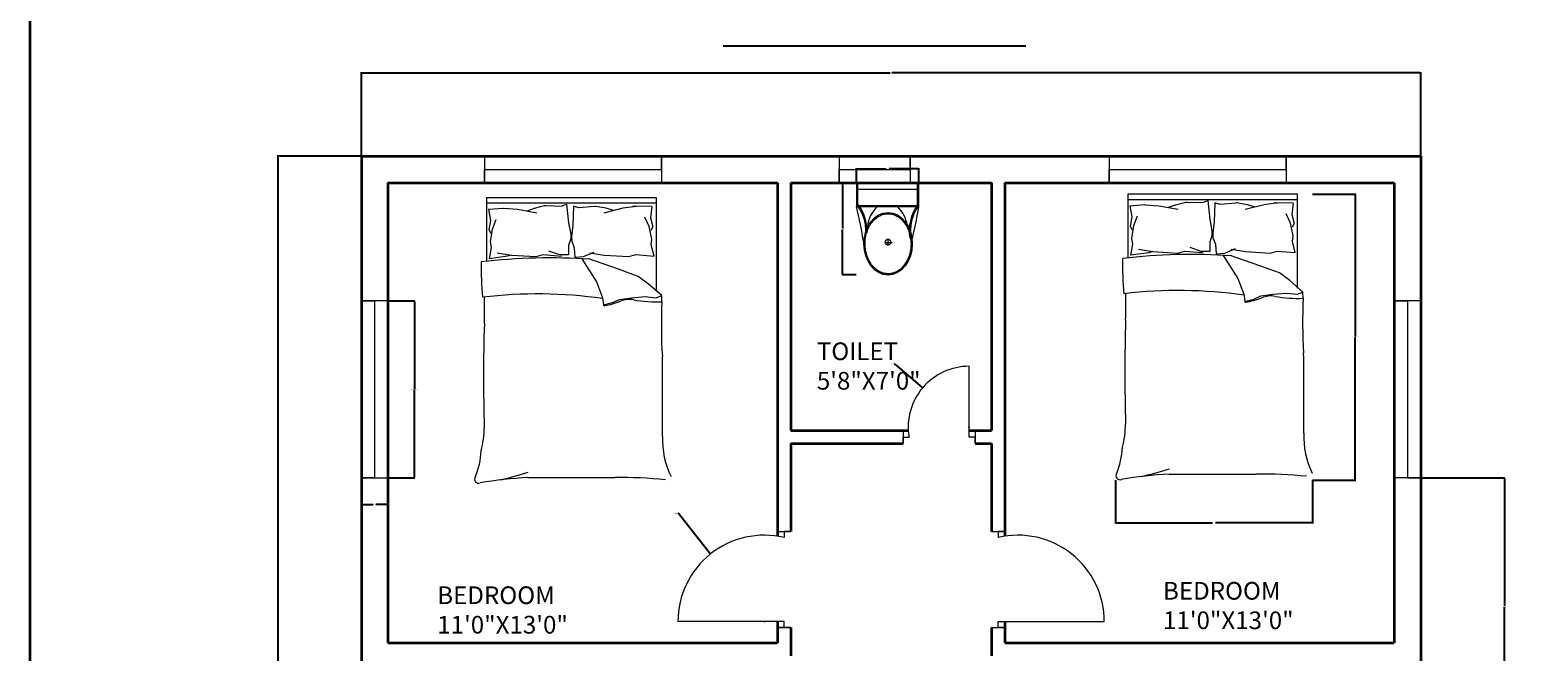
# Model space of a CAD drawing. Units: inches. Extents: x 1832 to 2989, y 1644 to 2902.
# Tile 3 of 8: x 1832 to 2343, y 2061 to 2272. Entities that reach past the tile are written whole.
import ezdxf

# ---------------------------------------------------------------- set-up
doc = ezdxf.new("R2010")
doc.units = ezdxf.units.IN
for name, color, linetype, lineweight in [('A-ANNO-DIMS', 2, 'Continuous', 18), ('A-ANNO-TEXT', 7, 'Continuous', 25), ('A-ANNO-TTLB', 7, 'Continuous', 35), ('A-AREA-IDEN', 7, 'Continuous', 18), ('A-DOOR', 3, 'Continuous', 18), ('A-FLOR-FIXT', 9, 'Continuous', 18), ('A-FURN', 8, 'Continuous', 18), ('A-GLAZ', 4, 'Continuous', 18), ('A-WALL', 7, 'Continuous', 35)]:
    doc.layers.add(name, color=color, linetype=linetype, lineweight=lineweight)
doc.styles.get("Standard").update_dxf_attribs({"font": 'arial.ttf'})
doc.dimstyles.get("Standard").update_dxf_attribs({"dimtxt": 0.18, "dimasz": 0.18, "dimexe": 0.18, "dimexo": 0.0625, "dimgap": 0.09, "dimtad": 0, "dimtih": 1, "dimtoh": 1, "dimdec": 4, "dimzin": 0, "dimdsep": 46, "dimtxsty": 'Standard', "dimcen": 0.09, "dimadec": 0, "dimazin": 0, "dimtfac": 1, "dimtdec": 4, "dimtofl": 0, "dimtmove": 0, "dimatfit": 3, "dimfxl": 1, "dimtolj": 1, "dimtzin": 0, "dimarcsym": 0})

# ---------------------------------------------------------------- blocks, each defined once
blk = doc.blocks.new('A$C31115884')
for p, q in [((258, 466), (258, 523)), ((283, 498), (223, 498)), ((0, 200), (0, 0)), ((520, 200), (0, 200)), ((10, 190), (10, 10)), ((510, 190), (10, 190)), ((510, 10), (510, 190)), ((520, 0), (520, 200)), ((510, 54), (0, 54)), ((10, 10), (510, 10)), ((0, 0), (520, 0))]:
    blk.add_line(p, q)
blk.add_circle((256, 496), 23.6)
for centre, radius, start, end in [((2778, -205), 2807, 165.4549, 171.7133), ((-295, 403), 365, 324.2091, 9.3499), ((-295, 403), 375, 324.2091, 9.3499), ((139, 406), 293, 315.8436, 2.6563), ((806, 403), 375, 179.2036, 215.7909), ((806, 403), 365, 170.6501, 215.7909), ((3237, 905), 2807, 188.2867, 194.5451), ((384, 406), 293, 190.2774, 224.1564)]:
    blk.add_arc(centre, radius, start, end)
blk.add_ellipse((256, 510), major_axis=(0, -261), ratio=0.772727)
blk.add_open_spline([(256, 259), (263, 259), (270, 260), (288, 262), (299, 265), (320, 273), (330, 278), (350, 291), (360, 299), (378, 316), (386, 326), (402, 347), (409, 358), (421, 383), (427, 395), (436, 422), (440, 436), (445, 465), (447, 480), (448, 509), (448, 524), (445, 553), (443, 568), (436, 596), (432, 610), (422, 636), (416, 649), (402, 672), (395, 683), (379, 703), (370, 712), (351, 728), (341, 735), (321, 746), (310, 751), (289, 757), (278, 759), (256, 761), (245, 761), (223, 757), (212, 754), (191, 746), (181, 741), (161, 728), (151, 720), (133, 703), (125, 693), (110, 672), (103, 660), (90, 636), (85, 623), (76, 596), (72, 582), (67, 553), (66, 538), (64, 509), (65, 494), (68, 465), (70, 450), (77, 422), (81, 408), (91, 382), (97, 370), (111, 346), (118, 335), (135, 316), (144, 307), (162, 291), (172, 284), (193, 273), (203, 269), (225, 262), (236, 260), (250, 259), (253, 259), (256, 259)], degree=3, knots=[0, 0, 0, 0, 0.110105, 0.110105, 0.285049, 0.285049, 0.459994, 0.459994, 0.634938, 0.634938, 0.809882, 0.809882, 0.984827, 0.984827, 1.159771, 1.159771, 1.334715, 1.334715, 1.50966, 1.50966, 1.684604, 1.684604, 1.859549, 1.859549, 2.034493, 2.034493, 2.209437, 2.209437, 2.384382, 2.384382, 2.559326, 2.559326, 2.73427, 2.73427, 2.909215, 2.909215, 3.084159, 3.084159, 3.259103, 3.259103, 3.434048, 3.434048, 3.608992, 3.608992, 3.783936, 3.783936, 3.958881, 3.958881, 4.133825, 4.133825, 4.30877, 4.30877, 4.483714, 4.483714, 4.658658, 4.658658, 4.833603, 4.833603, 5.008547, 5.008547, 5.183491, 5.183491, 5.358436, 5.358436, 5.53338, 5.53338, 5.708324, 5.708324, 5.883269, 5.883269, 6.058213, 6.058213, 6.233158, 6.233158, 6.283185, 6.283185, 6.283185, 6.283185])
blk = doc.blocks.new('BED-DOUBLE')
for p, q in [((4.17, 75.16), (4.17, 96.88)), ((4.17, 96.88), (61.46, 96.88)), ((4.17, 95.04), (61.46, 95.04)), ((4.67, 92.9), (5.36, 89.09)), ((4.68, 92.87), (9.81, 93.27)), ((9.81, 93.27), (9.93, 93.25)), ((9.93, 93.25), (14.52, 92.9)), ((14.52, 92.9), (21.1, 91.69)), ((17.81, 92.38), (20.24, 93.25)), ((20.24, 93.25), (23.7, 94.11)), ((23.7, 94.11), (24.09, 94.11)), ((24.09, 94.11), (29.42, 93.94)), ((29.42, 93.94), (31.15, 94.63)), ((31.15, 94.63), (31.84, 88.22)), ((33.54, 93.89), (33.25, 87.44)), ((35.31, 93.3), (33.54, 93.89)), ((40.62, 93.81), (35.31, 93.3)), ((41.01, 93.83), (40.62, 93.81)), ((44.52, 93.19), (41.01, 93.83)), ((50.25, 93.2), (43.75, 91.57)), ((47, 92.47), (44.52, 93.19)), ((54.8, 93.83), (50.25, 93.2)), ((60.08, 93.81), (53.6, 93.93)), ((53.6, 93.93), (54.8, 93.83)), ((60.08, 93.81), (59.62, 89.96)), ((61.46, 96.88), (61.46, 64.97)), ((5.36, 89.09), (4.84, 85.97)), ((6.06, 86.14), (7.27, 89.43)), ((31.84, 88.22), (32.54, 84.41)), ((33.25, 87.44), (32.8, 83.6)), ((59.12, 86.98), (57.7, 90.19)), ((60.08, 82.7), (59.12, 86.98)), ((59.62, 89.96), (60.34, 86.88)), ((60.34, 86.88), (59.72, 85.63)), ((4.84, 85.97), (5.54, 84.75)), ((5.36, 81.81), (6.06, 86.14)), ((5.71, 79.9), (5.36, 81.81)), ((32.54, 82.85), (31.84, 80.59)), ((32.54, 84.41), (32.54, 82.85)), ((32.8, 83.6), (32.89, 82.04)), ((32.89, 82.04), (33.73, 79.83)), ((59.85, 80.77), (60.08, 82.7)), ((5.02, 76.09), (5.71, 79.9)), ((11.13, 76.95), (5.02, 76.09)), ((7.65, 78.14), (12.49, 77.34)), ((12.49, 77.34), (11.13, 76.95)), ((12.49, 77.34), (20.89, 76.82)), ((20.89, 76.82), (23.24, 77.49)), ((23.24, 77.49), (29.39, 77.01)), ((28.9, 77.38), (25.13, 78.69)), ((31.84, 77.38), (28.9, 77.38)), ((31.84, 80.59), (31.84, 77.38)), ((33.73, 79.83), (33.93, 76.62)), ((33.93, 76.62), (36.87, 76.81)), ((36.87, 76.81), (40.55, 78.35)), ((39.04, 78.14), (43.88, 77.34)), ((43.88, 77.34), (52.28, 76.82)), ((52.28, 76.82), (54.63, 77.49)), ((54.63, 77.49), (60.78, 77.01)), ((60.78, 77.01), (59.85, 80.77)), ((36.28, 76.04), (41.3, 68.25)), ((48.73, 72.52), (38.73, 76.04)), ((55.41, 70.11), (48.73, 72.52)), ((41.3, 68.25), (43.34, 62.87)), ((58.94, 67.51), (55.41, 70.11)), ((63.38, 63.61), (58.94, 67.51)), ((43.34, 62.87), (43.72, 60.46)), ((46.69, 61.2), (49.1, 62.31)), ((49.1, 62.31), (53.18, 62.87)), ((53.18, 62.87), (57.83, 63.24)), ((57.83, 63.24), (61.54, 62.87)), ((61.54, 62.87), (63.38, 63.61)), ((63.48, 61.52), (63.38, 63.61, 4.64)), ((43.72, 60.46), (46.69, 61.2)), ((18.06, 1.87), (47.57, 1.87))]:
    blk.add_line(p, q)
for centre, radius, start, end in [((102.1, 72.78), 99.87, 178.7218, 185.604), ((25.61, -121.38), 197.77, 86.0865, 96.7821), ((21.29, -90.53), 154.68, 81.7845, 96.9006), ((-200.58, 59.5), 203.94, 358.4762, 1.0082), ((37.35, 95.1), 35.55, 280.6617, 289.8806), ((52.44, 54.84), 7.46, 78.6608, 113.7384), ((61.54, 104.86), 43.38, 259.8763, 272.5657), ((218.51, 53.34), 155.25, 176.9791, 183.8365), ((43.92, 60.38), 0.221, 160.2464, 271.1377), ((581.23, 36.2), 578.22, 178.22771, 181.71854), ((-5405.34, 15.57), 5469.02, 0.00217, 0.28689), ((-32.25, 19.53), 35.53, 346.0648, 358.9113), ((91.3, 14.55), 27.65, 177.4714, 206.4681), ((-25.96, 12.63), 28.25, 337.9751, 356.652), ((1.31, 1.31), 1.31, 146.1736, 293.4781), ((25.69, -143.9), 145.97, 92.9958, 99.4091), ((-20.64, 125.3), 127.63, 283.3832, 287.7053), ((49.34, -157.61), 159.5, 84.4998, 90.6351)]:
    blk.add_arc(centre, radius, start, end)
blk = doc.blocks.new('WIN-PLAN-60IN')
for p, q in [((0, 9), (0, 0)), ((60, 4.5), (60, 9)), ((60, 9), (60, 0)), ((0, 0), (0, 4.5)), ((0, 4.5), (60, 4.5))]:
    blk.add_line(p, q)
blk = doc.blocks.new('WIN-PLAN-60IN-2')
for p, q in [((9, 60), (0, 60)), ((0, 60), (4.5, 60)), ((4.5, 60), (4.5, 0)), ((4.5, 0), (0, 0)), ((0, 0), (9, 0))]:
    blk.add_line(p, q)
blk = doc.blocks.new('WIN-PLAN-24IN')
for p, q in [((0, 9), (0, 0)), ((24, 4.5), (24, 9)), ((24, 9), (24, 0)), ((0, 0), (0, 4.5)), ((0, 4.5), (24, 4.5))]:
    blk.add_line(p, q)
blk = doc.blocks.new('DOOR-PLAN-BEDROOM-L')
for p, q in [((33.75, 32.55), (38.25, 32.55)), ((38.25, 32.55), (36, 32.55)), ((36, 32.55), (36, 30.55)), ((36, 2), (0, 2)), ((33.75, 0), (38.25, 0)), ((38.25, 0), (33.75, 0)), ((33.75, 0), (36, 0)), ((36, 0), (36, 2))]:
    blk.add_line(p, q)
blk.add_arc((29.32, 2), 29.32, 76.8389, 180)
blk = doc.blocks.new('DOOR-PLAN-BATH')
for p, q in [((22.39, 2.25), (22.39, 26.25)), ((0, 4.5), (0, 0)), ((0, 0), (0, 2.25)), ((0, 2.25), (2, 2.25)), ((24.39, 2.25), (22.39, 2.25)), ((24.39, 4.5), (24.39, 0)), ((24.39, 0), (24.39, 2.25))]:
    blk.add_line(p, q)
blk.add_arc((22.39, 5.59), 20.66, 90, 189.2955)
blk = doc.blocks.new('DOOR-PLAN-BEDROOM-R')
for p, q in [((0, 32.55), (4.5, 32.55)), ((4.5, 32.55), (2.25, 32.55)), ((2.25, 32.55), (2.25, 30.55)), ((0, 0), (4.5, 0)), ((2.25, 0), (2.25, 2)), ((2.25, 2), (38.25, 2)), ((4.5, 0), (2.25, 0))]:
    blk.add_line(p, q)
blk.add_arc((8.93, 2), 29.32, 0, 103.1611)
blk = doc.blocks.new('*D25')
at = {"layer": 'A-ANNO-DIMS', "color": 0, "lineweight": -2, "transparency": 16777216}
for p, q in [((2266.19, 2216.33), (2280.86, 2216.33)), ((2280.68, 2216.15), (2280.68, 2168.02)), ((2280.68, 2119.51), (2280.68, 2167.65)), ((2266.19, 2119.33), (2280.86, 2119.33))]:
    blk.add_line(p, q, dxfattribs=at)
at = {"layer": 'A-ANNO-DIMS', "color": 0, "transparency": 16777216}
for points in [[(2280.65, 2216.15), (2280.71, 2216.15), (2280.68, 2216.33)], [(2280.65, 2119.51), (2280.71, 2119.51), (2280.68, 2119.33)]]:
    blk.add_solid(points, dxfattribs=at)
at = {"layer": 'Defpoints', "color": 0, "transparency": 16777216}
for p in [(2266.13, 2216.33), (2280.68, 2216.33), (2266.13, 2119.33)]:
    blk.add_point(p, dxfattribs=at)
at = {"layer": 'A-ANNO-DIMS', "color": 0, "transparency": 16777216, "insert": (2280.68, 2167.83), "char_height": 0.18, "attachment_point": 5}
blk.add_mtext('\\A1;DOUBLE BED 97 TYP.', dxfattribs=at)
blk = doc.blocks.new('*D26')
at = {"layer": 'A-ANNO-DIMS', "color": 0, "lineweight": -2, "transparency": 16777216}
for p, q in [((2199.47, 2119.27), (2199.47, 2104.6)), ((2266.13, 2119.27), (2266.13, 2104.6)), ((2199.65, 2104.78), (2232.27, 2104.78)), ((2265.95, 2104.78), (2233.33, 2104.78))]:
    blk.add_line(p, q, dxfattribs=at)
at = {"layer": 'A-ANNO-DIMS', "color": 0, "transparency": 16777216}
for points in [[(2199.65, 2104.81), (2199.65, 2104.75), (2199.47, 2104.78)], [(2265.95, 2104.81), (2265.95, 2104.75), (2266.13, 2104.78)]]:
    blk.add_solid(points, dxfattribs=at)
at = {"layer": 'Defpoints', "color": 0, "transparency": 16777216}
for p in [(2199.47, 2119.33), (2266.13, 2119.33), (2266.13, 2104.78)]:
    blk.add_point(p, dxfattribs=at)
at = {"layer": 'A-ANNO-DIMS', "color": 0, "transparency": 16777216, "insert": (2232.8, 2104.78), "char_height": 0.18, "attachment_point": 5}
blk.add_mtext('\\A1;67 TYP.', dxfattribs=at)
blk = doc.blocks.new('*D27')
at = {"layer": 'A-ANNO-DIMS', "color": 0, "lineweight": -2, "transparency": 16777216}
for p, q in [((2111.57, 2220.17), (2106.76, 2220.17)), ((2106.94, 2219.99), (2106.94, 2204.7)), ((2106.94, 2189.05), (2106.94, 2204.34)), ((2111.57, 2188.87), (2106.76, 2188.87))]:
    blk.add_line(p, q, dxfattribs=at)
at = {"layer": 'A-ANNO-DIMS', "color": 0, "transparency": 16777216}
for points in [[(2106.91, 2219.99), (2106.97, 2219.99), (2106.94, 2220.17)], [(2106.91, 2189.05), (2106.97, 2189.05), (2106.94, 2188.87)]]:
    blk.add_solid(points, dxfattribs=at)
at = {"layer": 'Defpoints', "color": 0, "transparency": 16777216}
for p in [(2111.64, 2220.17), (2106.94, 2188.87), (2111.64, 2188.87)]:
    blk.add_point(p, dxfattribs=at)
at = {"layer": 'A-ANNO-DIMS', "color": 0, "transparency": 16777216, "insert": (2106.94, 2204.52), "char_height": 0.18, "attachment_point": 5}
blk.add_mtext('\\A1;WC 31 TYP.', dxfattribs=at)
blk = doc.blocks.new('*D28')
at = {"layer": 'A-ANNO-DIMS', "color": 0, "lineweight": -2, "transparency": 16777216}
for p, q in [((2111.64, 2220.24), (2111.64, 2225.05)), ((2111.82, 2224.87), (2121.67, 2224.87)), ((2132.58, 2224.87), (2122.73, 2224.87)), ((2132.76, 2220.24), (2132.76, 2225.05))]:
    blk.add_line(p, q, dxfattribs=at)
at = {"layer": 'A-ANNO-DIMS', "color": 0, "transparency": 16777216}
for points in [[(2111.82, 2224.9), (2111.82, 2224.84), (2111.64, 2224.87)], [(2132.58, 2224.9), (2132.58, 2224.84), (2132.76, 2224.87)]]:
    blk.add_solid(points, dxfattribs=at)
at = {"layer": 'Defpoints', "color": 0, "transparency": 16777216}
for p in [(2111.64, 2224.87), (2111.64, 2220.17), (2132.76, 2220.17)]:
    blk.add_point(p, dxfattribs=at)
at = {"layer": 'A-ANNO-DIMS', "color": 0, "transparency": 16777216, "insert": (2122.2, 2224.87), "char_height": 0.18, "attachment_point": 5}
blk.add_mtext('\\A1;21 TYP.', dxfattribs=at)
blk = doc.blocks.new('*D51')
at = {"layer": 'A-ANNO-DIMS', "color": 0, "lineweight": -2, "transparency": 16777216}
for p, q in [((1952.95, 2180.08), (1962.07, 2180.08)), ((1961.89, 2179.9), (1961.89, 2150.27)), ((1961.89, 2120.26), (1961.89, 2149.9)), ((1952.95, 2120.08), (1962.07, 2120.08))]:
    blk.add_line(p, q, dxfattribs=at)
at = {"layer": 'A-ANNO-DIMS', "color": 0, "transparency": 16777216}
for points in [[(1961.86, 2179.9), (1961.92, 2179.9), (1961.89, 2180.08)], [(1961.86, 2120.26), (1961.92, 2120.26), (1961.89, 2120.08)]]:
    blk.add_solid(points, dxfattribs=at)
at = {"layer": 'Defpoints', "color": 0, "transparency": 16777216}
for p in [(1952.89, 2180.08), (1961.89, 2180.08), (1952.89, 2120.08)]:
    blk.add_point(p, dxfattribs=at)
at = {"layer": 'A-ANNO-DIMS', "color": 0, "transparency": 16777216, "insert": (1961.89, 2150.08), "char_height": 0.18, "attachment_point": 5}
blk.add_mtext('\\A1;SIDE WINDOW 60 TYP.', dxfattribs=at)
blk = doc.blocks.new('*D52')
at = {"layer": 'A-ANNO-DIMS', "color": 0, "lineweight": -2, "transparency": 16777216}
for p, q in [((1943.89, 2120.02), (1943.89, 2110.9)), ((1952.89, 2120.02), (1952.89, 2110.9)), ((1944.07, 2111.08), (1947.93, 2111.08)), ((1952.71, 2111.08), (1948.85, 2111.08))]:
    blk.add_line(p, q, dxfattribs=at)
at = {"layer": 'A-ANNO-DIMS', "color": 0, "transparency": 16777216}
for points in [[(1944.07, 2111.11), (1944.07, 2111.05), (1943.89, 2111.08)], [(1952.71, 2111.11), (1952.71, 2111.05), (1952.89, 2111.08)]]:
    blk.add_solid(points, dxfattribs=at)
at = {"layer": 'Defpoints', "color": 0, "transparency": 16777216}
for p in [(1943.89, 2120.08), (1952.89, 2120.08), (1952.89, 2111.08)]:
    blk.add_point(p, dxfattribs=at)
at = {"layer": 'A-ANNO-DIMS', "color": 0, "transparency": 16777216, "insert": (1948.39, 2111.08), "char_height": 0.18, "attachment_point": 5}
blk.add_mtext('\\A1;9 TYP.', dxfattribs=at)
blk = doc.blocks.new('*D71')
at = {"layer": 'A-ANNO-DIMS', "color": 0, "lineweight": -2, "transparency": 16777216}
for p, q in [((1943.89, 2229.24), (1943.89, 2257.65)), ((1944.07, 2257.47), (2123.1, 2257.47)), ((2302.71, 2257.47), (2123.68, 2257.47)), ((2302.89, 2229.24), (2302.89, 2257.65))]:
    blk.add_line(p, q, dxfattribs=at)
at = {"layer": 'A-ANNO-DIMS', "color": 0, "transparency": 16777216}
for points in [[(1944.07, 2257.5), (1944.07, 2257.44), (1943.89, 2257.47)], [(2302.71, 2257.5), (2302.71, 2257.44), (2302.89, 2257.47)]]:
    blk.add_solid(points, dxfattribs=at)
at = {"layer": 'Defpoints', "color": 0, "transparency": 16777216}
for p in [(2302.89, 2257.47), (1943.89, 2229.17), (2302.89, 2229.17)]:
    blk.add_point(p, dxfattribs=at)
at = {"layer": 'A-ANNO-DIMS', "color": 0, "transparency": 16777216, "insert": (2123.39, 2257.47), "char_height": 0.18, "attachment_point": 5}
blk.add_mtext('\\A1;359', dxfattribs=at)
blk = doc.blocks.new('*D72')
at = {"layer": 'A-ANNO-DIMS', "color": 0, "lineweight": -2, "transparency": 16777216}
for p, q in [((1943.83, 2229.17), (1915.41, 2229.17)), ((1915.59, 2228.99), (1915.59, 1975.53)), ((1915.59, 1721.7), (1915.59, 1975.17)), ((2089.33, 1721.52), (1915.41, 1721.52))]:
    blk.add_line(p, q, dxfattribs=at)
at = {"layer": 'A-ANNO-DIMS', "color": 0, "transparency": 16777216}
for points in [[(1915.56, 2228.99), (1915.62, 2228.99), (1915.59, 2229.17)], [(1915.56, 1721.7), (1915.62, 1721.7), (1915.59, 1721.52)]]:
    blk.add_solid(points, dxfattribs=at)
at = {"layer": 'Defpoints', "color": 0, "transparency": 16777216}
for p in [(1915.59, 2229.17), (1943.89, 2229.17), (2089.39, 1721.52)]:
    blk.add_point(p, dxfattribs=at)
at = {"layer": 'A-ANNO-DIMS', "color": 0, "transparency": 16777216, "insert": (1915.59, 1975.35), "char_height": 0.18, "attachment_point": 5}
blk.add_mtext('\\A1;507.6', dxfattribs=at)
blk = doc.blocks.new('*D74')
at = {"layer": 'A-ANNO-DIMS', "color": 0, "lineweight": -2, "transparency": 16777216}
for p, q in [((2302.95, 2120.08), (2331.37, 2120.08)), ((2331.19, 2119.9), (2331.19, 2076.73)), ((2331.19, 2033.19), (2331.19, 2076.36)), ((2302.95, 2033.01), (2331.37, 2033.01))]:
    blk.add_line(p, q, dxfattribs=at)
at = {"layer": 'A-ANNO-DIMS', "color": 0, "transparency": 16777216}
for points in [[(2331.16, 2119.9), (2331.22, 2119.9), (2331.19, 2120.08)], [(2331.16, 2033.19), (2331.22, 2033.19), (2331.19, 2033.01)]]:
    blk.add_solid(points, dxfattribs=at)
at = {"layer": 'Defpoints', "color": 0, "transparency": 16777216}
for p in [(2302.89, 2120.08), (2331.19, 2120.08), (2302.89, 2033.01)]:
    blk.add_point(p, dxfattribs=at)
at = {"layer": 'A-ANNO-DIMS', "color": 0, "transparency": 16777216, "insert": (2331.19, 2076.55), "char_height": 0.18, "attachment_point": 5}
blk.add_mtext('\\A1;87.08', dxfattribs=at)
blk = doc.blocks.new('*D122')
at = {"layer": 'A-ANNO-DIMS', "color": 0, "lineweight": -2, "transparency": 16777216}
for p, q in [((2051.13, 2108.07), (2051.31, 2108.07)), ((2051.31, 2108.07), (2062.13, 2094.43)), ((2080.37, 2071.31), (2080.55, 2071.31)), ((2080.46, 2071.22), (2080.46, 2071.4))]:
    blk.add_line(p, q, dxfattribs=at)
at = {"layer": 'A-ANNO-DIMS', "color": 0, "transparency": 16777216}
blk.add_solid([(2062.15, 2094.45), (2062.11, 2094.41), (2062.24, 2094.29)], dxfattribs=at)
at = {"layer": 'Defpoints', "color": 0, "transparency": 16777216}
for p in [(2062.24, 2094.29), (2080.46, 2071.31)]:
    blk.add_point(p, dxfattribs=at)
at = {"layer": 'A-ANNO-DIMS', "color": 0, "transparency": 16777216, "insert": (2050.38, 2108.07), "char_height": 0.18, "attachment_point": 5}
blk.add_mtext('\\A1;2X R29.323', dxfattribs=at)
blk = doc.blocks.new('*D126')
at = {"layer": 'A-ANNO-DIMS', "color": 0, "lineweight": -2, "transparency": 16777216}
for p, q in [((2124.48, 2158.67), (2124.66, 2158.67)), ((2124.66, 2158.67), (2133.97, 2150.76)), ((2149.77, 2137.26), (2149.95, 2137.26)), ((2149.86, 2137.17), (2149.86, 2137.35))]:
    blk.add_line(p, q, dxfattribs=at)
at = {"layer": 'A-ANNO-DIMS', "color": 0, "transparency": 16777216}
blk.add_solid([(2133.99, 2150.78), (2133.95, 2150.73), (2134.11, 2150.64)], dxfattribs=at)
at = {"layer": 'Defpoints', "color": 0, "transparency": 16777216}
for p in [(2134.11, 2150.64), (2149.86, 2137.26)]:
    blk.add_point(p, dxfattribs=at)
at = {"layer": 'A-ANNO-DIMS', "color": 0, "transparency": 16777216, "insert": (2123.93, 2158.67), "char_height": 0.18, "attachment_point": 5}
blk.add_mtext('\\A1;R20.662', dxfattribs=at)

msp = doc.modelspace()

# ---------------------------------------------------------------- linework, layer by layer
at = {"layer": 'A-ANNO-TEXT'}
msp.add_line((2066.5463, 2266.5968), (2169.0774, 2266.5968), dxfattribs=at)
at = {"layer": 'A-ANNO-TTLB'}
msp.add_lwpolyline([(1831.6677, 2901.9044), (2988.9144, 2901.9044), (2988.9144, 1643.5851), (1831.6677, 1643.5851)], close=True, dxfattribs=at)
at = {"layer": 'A-WALL'}
for p, q in [((1943.8904, 2229.1726), (1943.8904, 1750.6726)), ((1943.8904, 2229.1726), (1943.8904, 1750.6726)), ((1943.8904, 2229.1726), (1943.8904, 1750.6726)), ((1943.8904, 2229.1726), (2302.8904, 2229.1726)), ((2302.8904, 2229.1726), (2302.8904, 1846.6726)), ((1952.8904, 2220.1726), (2084.8904, 2220.1726)), ((1952.8904, 2220.1726), (1952.8904, 2064.1726)), ((2084.8904, 2220.1726), (2084.8904, 2100.2994)), ((2089.3904, 2220.1726), (2089.3904, 2136.1726)), ((2089.3904, 2220.1726), (2157.3904, 2220.1726)), ((2157.3904, 2220.1726), (2157.3904, 2136.1726)), ((2161.8904, 2220.1726), (2161.8904, 2100.2994)), ((2161.8904, 2220.1726), (2293.8904, 2220.1726)), ((2293.8904, 2220.1726), (2293.8904, 2064.1726)), ((2089.3904, 2136.1726), (2129.2221, 2136.1726)), ((2149.8559, 2136.1726), (2157.3904, 2136.1726)), ((2089.3904, 2131.6726), (2127.4648, 2131.6726)), ((2089.3904, 2131.6726), (2089.3904, 2101.8652)), ((2151.8559, 2131.6726), (2157.3904, 2131.6726)), ((2157.3904, 2131.6726), (2157.3904, 2101.8652)), ((2084.8904, 2071.312), (2084.8904, 2064.1726)), ((2089.3904, 2069.312), (2089.3904, 2064.1726)), ((2157.3904, 2069.312), (2157.3904, 2064.1726)), ((2161.8904, 2071.312), (2161.8904, 2064.1726)), ((1952.8904, 2064.1726), (2084.8904, 2064.1726)), ((2089.3904, 2064.1726), (2089.3904, 2059.6726)), ((2157.3904, 2064.1726), (2157.3904, 2059.6726)), ((2161.8904, 2064.1726), (2293.8904, 2064.1726))]:
    msp.add_line(p, q, dxfattribs=at)

# ---------------------------------------------------------------- block references
at = {"layer": 'A-DOOR'}
for name, p in [('DOOR-PLAN-BATH', (2127.4648, 2131.6726)), ('DOOR-PLAN-BEDROOM-L', (2051.1404, 2069.312)), ('DOOR-PLAN-BEDROOM-R', (2157.3904, 2069.312))]:
    msp.add_blockref(name, p, dxfattribs=at)
at = {"layer": 'A-FLOR-FIXT', "xscale": 0.0406268506401408, "yscale": 0.0406268506401408, "zscale": 0.0406268506401408, "rotation": 179.9999999999998}
msp.add_blockref('A$C31115884', (2132.7619, 2220.1726), dxfattribs=at)
at = {"layer": 'A-FURN'}
for p in [(1982.2781, 2118.2871), (2199.576, 2119.4556)]:
    msp.add_blockref('BED-DOUBLE', p, dxfattribs=at)
at = {"layer": 'A-GLAZ'}
for name, p in [('WIN-PLAN-60IN', (1985.5719, 2220.1726)), ('WIN-PLAN-24IN', (2105.8148, 2220.1726)), ('WIN-PLAN-60IN', (2197.2452, 2220.1726)), ('WIN-PLAN-60IN-2', (1943.8904, 2120.0845))]:
    msp.add_blockref(name, p, dxfattribs=at)
at = {"layer": 'A-GLAZ', "rotation": 270.0000000000009}
msp.add_blockref('WIN-PLAN-60IN', (2293.8904, 2180.0845), dxfattribs=at)

# ---------------------------------------------------------------- texts
at = {"layer": 'A-AREA-IDEN', "char_height": 6, "attachment_point": 1}
for s, width, insert in [('TOILET\\P5\'8"X7\'0"', 105.822025, (2098.232, 2166.0016)), ('BEDROOM\\P11\'0"X13\'0"', 139.520271, (2215.5254, 2084.7768)), ('BEDROOM\\P11\'0"X13\'0"', 178.697106, (1969.6057, 2083.2683))]:
    msp.add_mtext_dynamic_manual_height_columns(s, width=width, gutter_width=12.5, heights=[0], dxfattribs=dict(at, insert=insert))

# ---------------------------------------------------------------- dimensions: what is measured, and where the dimension line sits
at = {"layer": 'A-ANNO-DIMS'}
dim = msp.add_linear_dim(base=(2302.8904, 2257.4726), p1=(1943.8904, 2229.1726), p2=(2302.8904, 2229.1726), dimstyle='Standard', override={"dimdec": 0, "dimlfac": 1, "dimrnd": 0, "dimzin": 0, "dimdsep": 46, "dimlunit": 2}, dxfattribs=at)
dim.commit()
dim.dimension.update_dxf_attribs({"geometry": '*D71', "text_midpoint": (2123.3904, 2257.4726)})
for base, p1, p2, override, picture, middle in [((1915.5904, 2229.1726), (2089.3904, 1721.5243), (1943.8904, 2229.1726), {"dimdec": 1, "dimlfac": 1, "dimrnd": 0, "dimzin": 0, "dimdsep": 46, "dimlunit": 2}, '*D72', (1915.5904, 1975.3484)), ((2331.1904, 2120.0845), (2302.8904, 2033.0074), (2302.8904, 2120.0845), {"dimdec": 2, "dimlfac": 1, "dimrnd": 0, "dimzin": 0, "dimdsep": 46, "dimlunit": 2}, '*D74', (2331.1904, 2076.546))]:
    dim = msp.add_linear_dim(base=base, p1=p1, p2=p2, angle=90, dimstyle='Standard', override=override, dxfattribs=at)
    dim.commit()
    dim.dimension.update_dxf_attribs({"geometry": picture, "text_midpoint": middle})
for base, p1, p2, angle, text, picture, middle in [((2111.636, 2224.8684), (2132.7619, 2220.1726), (2111.636, 2220.1726), 180, '<> TYP.', '*D28', (2122.199, 2224.8684)), ((2106.9401, 2188.8667), (2111.636, 2220.1726), (2111.636, 2188.8667), 270, 'WC <> TYP.', '*D27', (2106.9401, 2204.5196)), ((2280.6757, 2216.3316), (2266.1259, 2119.3329), (2266.1259, 2216.3316), 90, 'DOUBLE BED <> TYP.', '*D25', (2280.6757, 2167.8322)), ((1961.8904, 2180.0845), (1952.8904, 2120.0845), (1952.8904, 2180.0845), 90, 'SIDE WINDOW <> TYP.', '*D51', (1961.8904, 2150.0845))]:
    dim = msp.add_linear_dim(base=base, p1=p1, p2=p2, angle=angle, text=text, dimstyle='Standard', override={"dimdec": 0, "dimlfac": 1, "dimrnd": 0, "dimzin": 0, "dimdsep": 46, "dimlunit": 2}, dxfattribs=at)
    dim.commit()
    dim.dimension.update_dxf_attribs({"geometry": picture, "text_midpoint": middle})
dim = msp.add_radius_dim(center=(2149.8559, 2137.2601), mpoint=(2134.1099, 2150.6391), dimstyle='Standard', override={"dimdec": 3, "dimlfac": 1, "dimrnd": 0, "dimzin": 0, "dimdsep": 46, "dimlunit": 2}, dxfattribs=at)
dim.commit()
dim.dimension.update_dxf_attribs({"geometry": '*D126', "text_midpoint": (2123.9334, 2158.6665), "dimtype": 164})
for base, p1, p2, picture, middle in [((1952.8904, 2111.0845), (1943.8904, 2120.0845), (1952.8904, 2120.0845), '*D52', (1948.3904, 2111.0845)), ((2266.1259, 2104.783), (2199.4744, 2119.3329), (2266.1259, 2119.3329), '*D26', (2232.8001, 2104.783))]:
    dim = msp.add_linear_dim(base=base, p1=p1, p2=p2, text='<> TYP.', dimstyle='Standard', override={"dimdec": 0, "dimlfac": 1, "dimrnd": 0, "dimzin": 0, "dimdsep": 46, "dimlunit": 2}, dxfattribs=at)
    dim.commit()
    dim.dimension.update_dxf_attribs({"geometry": picture, "text_midpoint": middle})
dim = msp.add_radius_dim(center=(2080.4638, 2071.312), mpoint=(2062.2417, 2094.2863), text='2X <>', dimstyle='Standard', override={"dimdec": 3, "dimlfac": 1, "dimrnd": 0, "dimzin": 0, "dimdsep": 46, "dimlunit": 2}, dxfattribs=at)
dim.commit()
dim.dimension.update_dxf_attribs({"geometry": '*D122', "text_midpoint": (2050.3838, 2108.0709), "dimtype": 164})

doc.saveas('drawing.dxf')
